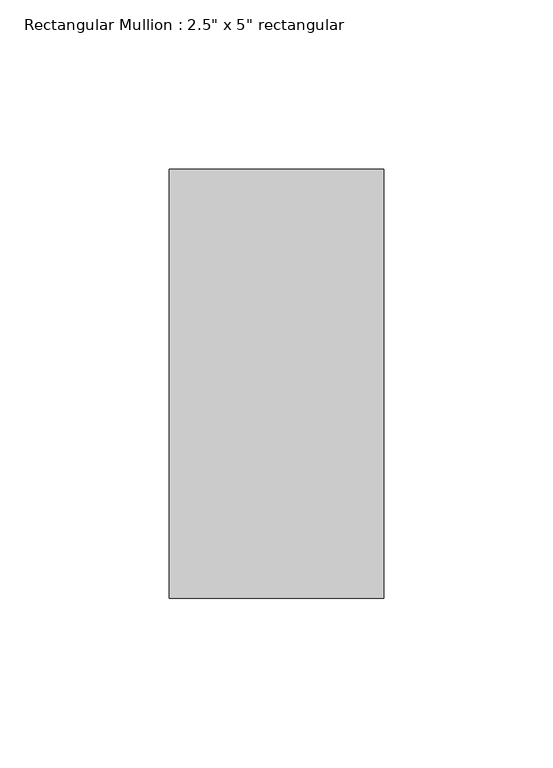
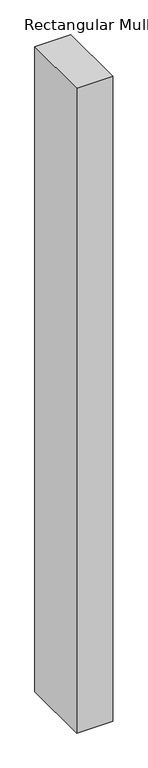
"""IFC4 building model written with IfcOpenShell, lengths in millimetres: member geometry."""

from ifc_helpers import new_model, si_unit, frame, origin, place, context, project, spatial, polyline, outline, extrude, source, transform, mapped, element, save


def member_3e1bda4a(model_context):
    return source(origin(), model_context, "Body", "SweptSolid", [
        extrude(outline(polyline([(0.0, 63.5), (0.0, -63.5), (-63.5, -63.5), (-63.5, 63.5), (0.0, 63.5)])), frame((0.0, 0.0, -1200.1500001), z_axis=(0.0, 0.0, 1.0), x_axis=(1.0, 0.0, 0.0)), (0.0, 0.0, 1.0), 1200.1500001),
    ])


if __name__ == "__main__":
    model = new_model("IFC4")
    model_context = context("Model", 3, world=origin())
    ifc_project = project(units=[si_unit("LENGTHUNIT", "METRE", prefix="MILLI")], contexts=[model_context])
    site = spatial("IfcSite", under=ifc_project)
    building = spatial("IfcBuilding", under=site)
    placement = place(None, origin())
    member_shape = member_3e1bda4a(model_context)
    element("IfcMember", 1, ObjectType="Rectangular Mullion : 2.5\" x 5\" rectangular", at=placement, inside=building, context=model_context, shape_type="MappedRepresentation", body=[
        mapped(member_shape, transform((0.0, 0.0, 0.0), x_axis=(1.0, 0.0, 0.0), y_axis=(0.0, 1.0, 0.0), z_axis=(0.0, 0.0, 1.0))),
    ])
    save(model, "model.ifc")

# Revit data of these elements
# Type "Rectangular Mullion : 2.5\" x 5\" rectangular"
#   built-in parameter 1007304 = 0.416667 (stored number, unit not read)
#   built-in parameter 1007301 = 0.104167 (stored number, unit not read)
#   built-in parameter 1007300 = 0.104167 (stored number, unit not read)
# Element 1 (IfcMember, "Rectangular Mullion : 2.5\" x 5\" rectangular")
#   Materials on its faces: "Aluminum"
# Materials
#   "Aluminum": class "Metal", colour RGB 247 247 247, transparency 0, Description = "Aluminum 6061", Cost = 0
